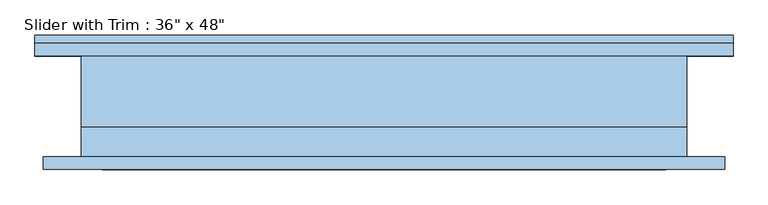
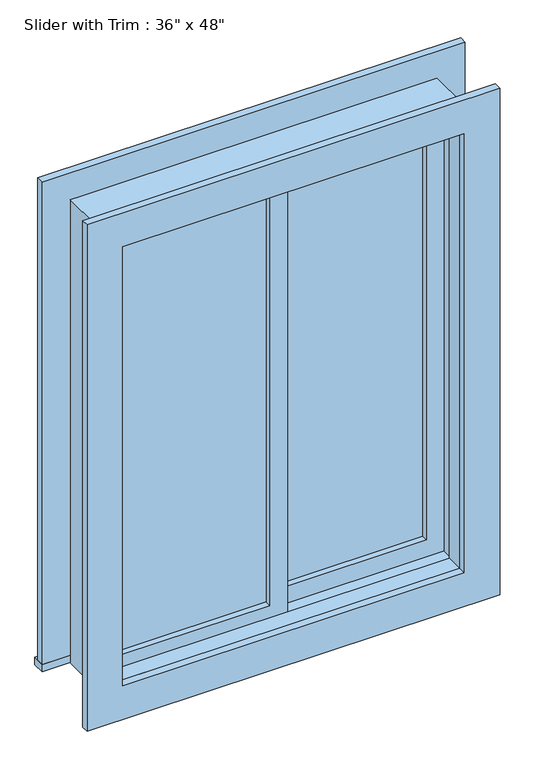
"""IFC4 building model written with IfcOpenShell, lengths in millimetres: window geometry."""

from ifc_helpers import new_model, si_unit, frame, origin, place, context, project, spatial, polyline, outline, extrude, source, transform, mapped, element, save


def window_99c3d43f(model_context):
    return source(origin(), model_context, "Body", "SweptSolid", [
        extrude(outline(polyline([(-393.7, -3.175), (-22.225, -3.175), (-22.225, -15.875), (-393.7, -15.875), (-393.7, -3.175)])), frame((0.0, 0.0, 977.9), z_axis=(0.0, 0.0, 1.0), x_axis=(1.0, 0.0, 0.0)), (0.0, 0.0, 1.0), 1092.2),
        extrude(outline(polyline([(2114.55, -438.15), (933.45, -438.15), (933.45, 22.225), (2114.55, 22.225), (2114.55, -438.15)]), holes=[polyline([(2070.1, -393.7), (2070.1, -22.225), (977.9, -22.225), (977.9, -393.7), (2070.1, -393.7)])]), frame((0.0, -31.75, 0.0), z_axis=(0.0, 1.0, 0.0), x_axis=(0.0, 0.0, 1.0)), (0.0, 0.0, 1.0), 44.45),
        extrude(outline(polyline([(-527.05, 107.95), (527.05, 107.95), (527.05, 76.2), (-527.05, 76.2), (-527.05, 107.95)])), frame((0.0, 0.0, 914.4), z_axis=(0.0, 0.0, 1.0), x_axis=(1.0, 0.0, 0.0)), (0.0, 0.0, 1.0), 19.05),
        extrude(outline(polyline([(2114.55, -438.15), (2114.55, 438.15), (933.45, 438.15), (933.45, 527.05), (2203.45, 527.05), (2203.45, -527.05), (933.45, -527.05), (933.45, -438.15), (2114.55, -438.15)])), frame((0.0, 76.2, 0.0), z_axis=(0.0, 1.0, 0.0), x_axis=(0.0, 0.0, 1.0)), (0.0, 0.0, 1.0), 19.05),
        extrude(outline(polyline([(2190.75, 514.35), (2190.75, -514.35), (857.25, -514.35), (857.25, 514.35), (2190.75, 514.35)]), holes=[polyline([(2101.85, 425.45), (946.15, 425.45), (946.15, -425.45), (2101.85, -425.45), (2101.85, 425.45)])]), frame((0.0, -95.25, 0.0), z_axis=(0.0, 1.0, 0.0), x_axis=(0.0, 0.0, 1.0)), (0.0, 0.0, 1.0), 19.05),
        extrude(outline(polyline([(393.7, 28.575), (22.225, 28.575), (22.225, 41.275), (393.7, 41.275), (393.7, 28.575)])), frame((0.0, 0.0, 977.9), z_axis=(0.0, 0.0, 1.0), x_axis=(1.0, 0.0, 0.0)), (0.0, 0.0, 1.0), 1092.2),
        extrude(outline(polyline([(2114.55, -22.225), (933.45, -22.225), (933.45, 438.15), (2114.55, 438.15), (2114.55, -22.225)]), holes=[polyline([(2070.1, 22.225), (2070.1, 393.7), (977.9, 393.7), (977.9, 22.225), (2070.1, 22.225)])]), frame((0.0, 12.7, 0.0), z_axis=(0.0, 1.0, 0.0), x_axis=(0.0, 0.0, 1.0)), (0.0, 0.0, 1.0), 44.45),
        extrude(outline(polyline([(2133.6, -457.2), (914.4, -457.2), (914.4, 457.2), (2133.6, 457.2), (2133.6, -457.2)]), holes=[polyline([(2101.85, -425.45), (2101.85, 425.45), (946.15, 425.45), (946.15, -425.45), (2101.85, -425.45)])]), frame((0.0, -76.2, 0.0), z_axis=(0.0, 1.0, 0.0), x_axis=(0.0, 0.0, 1.0)), (0.0, 0.0, 1.0), 44.45),
        extrude(outline(polyline([(2133.6, 457.2), (2133.6, -457.2), (914.4, -457.2), (914.4, 457.2), (2133.6, 457.2)]), holes=[polyline([(2114.55, 438.15), (933.45, 438.15), (933.45, -438.15), (2114.55, -438.15), (2114.55, 438.15)])]), frame((0.0, -31.75, 0.0), z_axis=(0.0, 1.0, 0.0), x_axis=(0.0, 0.0, 1.0)), (0.0, 0.0, 1.0), 107.95),
    ])


if __name__ == "__main__":
    model = new_model("IFC4")
    model_context = context("Model", 3, world=origin())
    ifc_project = project(units=[si_unit("LENGTHUNIT", "METRE", prefix="MILLI")], contexts=[model_context])
    site = spatial("IfcSite", under=ifc_project)
    building = spatial("IfcBuilding", under=site)
    placement = place(None, origin())
    window_shape = window_99c3d43f(model_context)
    element("IfcWindow", 1, ObjectType="Slider with Trim : 36\" x 48\"", at=placement, inside=building, context=model_context, shape_type="MappedRepresentation", body=[
        mapped(window_shape, transform((0.0, 0.0, 0.0), x_axis=(1.0, 0.0, 0.0), y_axis=(0.0, 1.0, 0.0), z_axis=(0.0, 0.0, 1.0))),
    ])
    save(model, "model.ifc")

# Revit data of these elements
# Type "Slider with Trim : 36\" x 48\""
#   Type Mark = "10"
#   Construction Type Id = "GSP4R"
#   Assembly Code = "B2020100"
#   Analytic Construction = "1/8 in Pilkington single glazing"
#   Visual Light Transmittance = 0.9
#   Solar Heat Gain Coefficient = 0.78
#   Heat Transfer Coefficient (U) = 0.6496 BTU/(h·ft²·°F)
#   Height = 4' - 0"
#   Default Sill Height = 3' - 0"
#   Trim Projection - Ext. = 0' - 0 3/4"
#   Trim Projection - Int. = 0' - 0 3/4"
#   Trim Width - Exterior = 0' - 3 1/2"
#   Trim Width - Interior = 0' - 3 1/2"
#   Width = 3' - 0"
#   Window Inset = 0' - 0 3/4"
#   Define Thermal Properties by = 1
#   Glass Pane Material = Glass
#   Sash Material = Sash
#   Trim Exterior Material = Trim
#   Trim Interior Material = Trim
#   Wall Closure = (empty or 0)
# Element 1 (IfcWindow, "Slider with Trim : 36\" x 48\"")
#   Materials on its faces: "Sash", "Trim", "Glass"
# Materials
#   "Glass": class "Glass", colour RGB 0 128 192, transparency 0.75, Description = "Soda Lime Glass", Cost = 0
#   "Sash": class "Wood", colour RGB 224 178 126, transparency 0
#   "Trim": class "Wood", colour RGB 224 178 126, transparency 0
